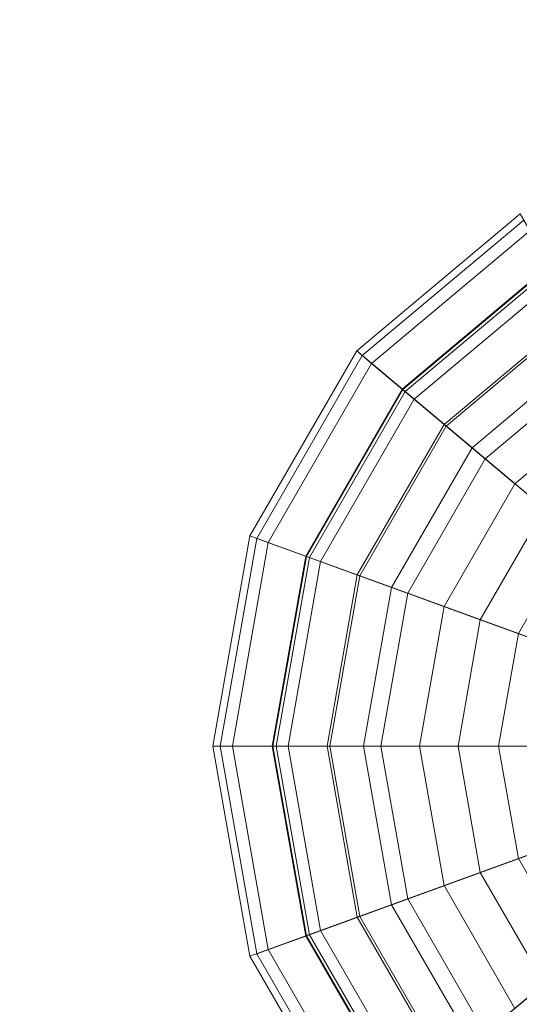
# Model space of a CAD drawing. Units: inches. Extents: x 375 to 1122, y 27 to 1069.
# Tile 109 of 155: x 731.282 to 732.383, y 872.701 to 874.871. Entities that reach past the tile are written whole.
import ezdxf

# ---------------------------------------------------------------- set-up
doc = ezdxf.new("R2010")
doc.units = ezdxf.units.IN
doc.layers.add('A-ANNO-DIMS', color=2, linetype='Continuous', lineweight=18)
doc.layers.add('Furniture', color=30, linetype='Continuous', lineweight=18)
doc.styles.get("Standard").update_dxf_attribs({"font": 'arial.ttf'})
doc.dimstyles.new('ISO-25', dxfattribs={"dimtxt": 12, "dimasz": 2.5, "dimexe": 1.5, "dimexo": 1.5, "dimtad": 1, "dimdec": 1, "dimlunit": 3, "dimtxsty": 'Standard', "dimblk": 'ARCHTICK', "dimcen": 2.5, "dimadec": 0, "dimazin": 0, "dimtfac": 1, "dimtdec": 1, "dimtmove": 0, "dimatfit": 3, "dimfxl": 1.5, "dimfxlon": 1, "dimarcsym": 0})

# ---------------------------------------------------------------- blocks, each defined once
blk = doc.blocks.new('A$C403C54AD')
for points in [[(1.597139, 1.185986, -0.04658), (1.626464, 1.202917, -0.043501), (1.626464, 1.202917, -0.043501), (1.604698, 1.176977, -0.04658)], [(1.604698, 1.176977, -0.04658), (1.626464, 1.202917, -0.043501), (1.626464, 1.202917, -0.043501), (1.614883, 1.171097, -0.04658)], [(1.614883, 1.171097, -0.04658), (1.626464, 1.202917, -0.043501), (1.626464, 1.202917, -0.043501), (1.626464, 1.169055, -0.04658)], [(1.64823, 1.176977, -0.04658), (1.626464, 1.202917, -0.043501), (1.626464, 1.202917, -0.043501), (1.65579, 1.185986, -0.04658)], [(1.638046, 1.171097, -0.04658), (1.626464, 1.202917, -0.043501), (1.626464, 1.202917, -0.043501), (1.64823, 1.176977, -0.04658)], [(1.626464, 1.169055, -0.04658), (1.626464, 1.202917, -0.043501), (1.626464, 1.202917, -0.043501), (1.638046, 1.171097, -0.04658)], [(1.620741, 1.196096, 0.042248), (1.614812, 1.189031, 0.048884), (1.620264, 1.185883, 0.048884), (1.623419, 1.19455, 0.042248)], [(1.62951, 1.19455, 0.042248), (1.632664, 1.185883, 0.048884), (1.638116, 1.189031, 0.048884), (1.632188, 1.196096, 0.042248)], [(1.614154, 1.19581, -0.040074), (1.599967, 1.187619, -0.043349), (1.606797, 1.179479, -0.043349), (1.617327, 1.192029, -0.040074)], [(1.635601, 1.192029, -0.040074), (1.646131, 1.179479, -0.043349), (1.652961, 1.187619, -0.043349), (1.638774, 1.19581, -0.040074)], [(1.613379, 1.187323, 0.046697), (1.61996, 1.195166, 0.03933), (1.623003, 1.193409, 0.03933), (1.619501, 1.183788, 0.046697)], [(1.633427, 1.183788, 0.046697), (1.629925, 1.193409, 0.03933), (1.632968, 1.195166, 0.03933), (1.63955, 1.187323, 0.046697)], [(1.623419, 1.19455, 0.042248), (1.620264, 1.185883, 0.048884), (1.626464, 1.18479, 0.048884), (1.626464, 1.194013, 0.042248)], [(1.626464, 1.194013, 0.042248), (1.626464, 1.18479, 0.048884), (1.632664, 1.185883, 0.048884), (1.62951, 1.19455, 0.042248)], [(1.610766, 1.193854, 0.048884), (1.605149, 1.190611, 0.058276), (1.610643, 1.184063, 0.058276), (1.614812, 1.189031, 0.048884)], [(1.619501, 1.183788, 0.046697), (1.623003, 1.193409, 0.03933), (1.626464, 1.192799, 0.03933), (1.626464, 1.18256, 0.046697)], [(1.626464, 1.18256, 0.046697), (1.626464, 1.192799, 0.03933), (1.629925, 1.193409, 0.03933), (1.633427, 1.183788, 0.046697)], [(1.638116, 1.189031, 0.048884), (1.642285, 1.184063, 0.058276), (1.64778, 1.190611, 0.058276), (1.642163, 1.193854, 0.048884)], [(1.602714, 1.189206, 0.056929), (1.608834, 1.192739, 0.046697), (1.613379, 1.187323, 0.046697), (1.608836, 1.18191, 0.056929)], [(1.644092, 1.18191, 0.056929), (1.63955, 1.187323, 0.046697), (1.644094, 1.192739, 0.046697), (1.650214, 1.189206, 0.056929)], [(1.617327, 1.192029, -0.040074), (1.606797, 1.179479, -0.043349), (1.616, 1.174166, -0.043349), (1.621603, 1.18956, -0.040074)], [(1.631326, 1.18956, -0.040074), (1.636929, 1.174166, -0.043349), (1.646131, 1.179479, -0.043349), (1.635601, 1.192029, -0.040074)], [(1.602589, 1.189133, 0.115599), (1.606995, 1.191677, 0.12581), (1.612014, 1.185696, 0.12581), (1.608743, 1.181798, 0.115599)], [(1.606995, 1.191677, 0.12581), (1.604329, 1.190138, 0.12581), (1.610035, 1.183338, 0.12581), (1.612014, 1.185696, 0.12581)], [(1.604329, 1.190138, 0.12581), (1.600002, 1.187639, 0.116404), (1.606823, 1.17951, 0.116404), (1.610035, 1.183338, 0.12581)], [(1.605149, 1.190611, 0.058276), (1.600725, 1.188057, 0.075423), (1.60736, 1.18015, 0.075423), (1.610643, 1.184063, 0.058276)], [(1.621603, 1.18956, -0.040074), (1.616, 1.174166, -0.043349), (1.626464, 1.172321, -0.043349), (1.626464, 1.188703, -0.040074)], [(1.626464, 1.188703, -0.040074), (1.626464, 1.172321, -0.043349), (1.636929, 1.174166, -0.043349), (1.631326, 1.18956, -0.040074)], [(1.598069, 1.186523, 0.074938), (1.602714, 1.189206, 0.056929), (1.608836, 1.18191, 0.056929), (1.605388, 1.1778, 0.074938)], [(1.600155, 1.187728, 0.102963), (1.602589, 1.189133, 0.115599), (1.608743, 1.181798, 0.115599), (1.606937, 1.179646, 0.102963)], [(1.614812, 1.189031, 0.048884), (1.610643, 1.184063, 0.058276), (1.618046, 1.179789, 0.058276), (1.620264, 1.185883, 0.048884)], [(1.632664, 1.185883, 0.048884), (1.634882, 1.179789, 0.058276), (1.642285, 1.184063, 0.058276), (1.638116, 1.189031, 0.048884)], [(1.600725, 1.188057, 0.075423), (1.600155, 1.187728, 0.102963), (1.606937, 1.179646, 0.102963), (1.60736, 1.18015, 0.075423)], [(1.599967, 1.187619, -0.043349), (1.597139, 1.185986, -0.04658), (1.604698, 1.176977, -0.04658), (1.606797, 1.179479, -0.043349)], [(1.600002, 1.187639, 0.116404), (1.597484, 1.186186, 0.10318), (1.604954, 1.177283, 0.10318), (1.606823, 1.17951, 0.116404)], [(1.608836, 1.18191, 0.056929), (1.613379, 1.187323, 0.046697), (1.619501, 1.183788, 0.046697), (1.617085, 1.177147, 0.056929)], [(1.635844, 1.177147, 0.056929), (1.633427, 1.183788, 0.046697), (1.63955, 1.187323, 0.046697), (1.644092, 1.18191, 0.056929)], [(1.597484, 1.186186, 0.10318), (1.598069, 1.186523, 0.074938), (1.605388, 1.1778, 0.074938), (1.604954, 1.177283, 0.10318)], [(1.620264, 1.185883, 0.048884), (1.618046, 1.179789, 0.058276), (1.626464, 1.178304, 0.058276), (1.626464, 1.18479, 0.048884)], [(1.626464, 1.18479, 0.048884), (1.626464, 1.178304, 0.058276), (1.634882, 1.179789, 0.058276), (1.632664, 1.185883, 0.048884)], [(1.608743, 1.181798, 0.115599), (1.612014, 1.185696, 0.12581), (1.618775, 1.181792, 0.12581), (1.617035, 1.177011, 0.115599)], [(1.612014, 1.185696, 0.12581), (1.610035, 1.183338, 0.12581), (1.617722, 1.178899, 0.12581), (1.618775, 1.181792, 0.12581)], [(1.634153, 1.181792, 0.12581), (1.635206, 1.178899, 0.12581), (1.642894, 1.183338, 0.12581), (1.640915, 1.185696, 0.12581)], [(1.635893, 1.177011, 0.115599), (1.634153, 1.181792, 0.12581), (1.640915, 1.185696, 0.12581), (1.644185, 1.181798, 0.115599)], [(1.610643, 1.184063, 0.058276), (1.60736, 1.18015, 0.075423), (1.616299, 1.174989, 0.075423), (1.618046, 1.179789, 0.058276)], [(1.617085, 1.177147, 0.056929), (1.619501, 1.183788, 0.046697), (1.626464, 1.18256, 0.046697), (1.626464, 1.175494, 0.056929)], [(1.626464, 1.175494, 0.056929), (1.626464, 1.18256, 0.046697), (1.633427, 1.183788, 0.046697), (1.635844, 1.177147, 0.056929)], [(1.634882, 1.179789, 0.058276), (1.636629, 1.174989, 0.075423), (1.645568, 1.18015, 0.075423), (1.642285, 1.184063, 0.058276)], [(1.610035, 1.183338, 0.12581), (1.606823, 1.17951, 0.116404), (1.616013, 1.174204, 0.116404), (1.617722, 1.178899, 0.12581)], [(1.635206, 1.178899, 0.12581), (1.636915, 1.174204, 0.116404), (1.646105, 1.17951, 0.116404), (1.642894, 1.183338, 0.12581)], [(1.605388, 1.1778, 0.074938), (1.608836, 1.18191, 0.056929), (1.617085, 1.177147, 0.056929), (1.61525, 1.172106, 0.074938)], [(1.606937, 1.179646, 0.102963), (1.608743, 1.181798, 0.115599), (1.617035, 1.177011, 0.115599), (1.616074, 1.174371, 0.102963)], [(1.617035, 1.177011, 0.115599), (1.618775, 1.181792, 0.12581), (1.626464, 1.180436, 0.12581), (1.626464, 1.175348, 0.115599)], [(1.618775, 1.181792, 0.12581), (1.617722, 1.178899, 0.12581), (1.626464, 1.177358, 0.12581), (1.626464, 1.180436, 0.12581)], [(1.626464, 1.180436, 0.12581), (1.626464, 1.177358, 0.12581), (1.635206, 1.178899, 0.12581), (1.634153, 1.181792, 0.12581)], [(1.626464, 1.175348, 0.115599), (1.626464, 1.180436, 0.12581), (1.634153, 1.181792, 0.12581), (1.635893, 1.177011, 0.115599)], [(1.637678, 1.172106, 0.074938), (1.635844, 1.177147, 0.056929), (1.644092, 1.18191, 0.056929), (1.64754, 1.1778, 0.074938)], [(1.636854, 1.174371, 0.102963), (1.635893, 1.177011, 0.115599), (1.644185, 1.181798, 0.115599), (1.645991, 1.179646, 0.102963)], [(1.60736, 1.18015, 0.075423), (1.606937, 1.179646, 0.102963), (1.616074, 1.174371, 0.102963), (1.616299, 1.174989, 0.075423)], [(1.636629, 1.174989, 0.075423), (1.636854, 1.174371, 0.102963), (1.645991, 1.179646, 0.102963), (1.645568, 1.18015, 0.075423)], [(1.606797, 1.179479, -0.043349), (1.604698, 1.176977, -0.04658), (1.614883, 1.171097, -0.04658), (1.616, 1.174166, -0.043349)], [(1.606823, 1.17951, 0.116404), (1.604954, 1.177283, 0.10318), (1.615019, 1.171472, 0.10318), (1.616013, 1.174204, 0.116404)], [(1.618046, 1.179789, 0.058276), (1.616299, 1.174989, 0.075423), (1.626464, 1.173197, 0.075423), (1.626464, 1.178304, 0.058276)], [(1.626464, 1.178304, 0.058276), (1.626464, 1.173197, 0.075423), (1.636629, 1.174989, 0.075423), (1.634882, 1.179789, 0.058276)], [(1.636915, 1.174204, 0.116404), (1.637909, 1.171472, 0.10318), (1.647974, 1.177283, 0.10318), (1.646105, 1.17951, 0.116404)], [(1.636929, 1.174166, -0.043349), (1.638046, 1.171097, -0.04658), (1.64823, 1.176977, -0.04658), (1.646131, 1.179479, -0.043349)], [(1.617722, 1.178899, 0.12581), (1.616013, 1.174204, 0.116404), (1.626464, 1.172361, 0.116404), (1.626464, 1.177358, 0.12581)], [(1.626464, 1.177358, 0.12581), (1.626464, 1.172361, 0.116404), (1.636915, 1.174204, 0.116404), (1.635206, 1.178899, 0.12581)], [(1.604954, 1.177283, 0.10318), (1.605388, 1.1778, 0.074938), (1.61525, 1.172106, 0.074938), (1.615019, 1.171472, 0.10318)], [(1.637909, 1.171472, 0.10318), (1.637678, 1.172106, 0.074938), (1.64754, 1.1778, 0.074938), (1.647974, 1.177283, 0.10318)], [(1.61525, 1.172106, 0.074938), (1.617085, 1.177147, 0.056929), (1.626464, 1.175494, 0.056929), (1.626464, 1.170129, 0.074938)], [(1.626464, 1.170129, 0.074938), (1.626464, 1.175494, 0.056929), (1.635844, 1.177147, 0.056929), (1.637678, 1.172106, 0.074938)], [(1.616074, 1.174371, 0.102963), (1.617035, 1.177011, 0.115599), (1.626464, 1.175348, 0.115599), (1.626464, 1.172539, 0.102963)], [(1.626464, 1.172539, 0.102963), (1.626464, 1.175348, 0.115599), (1.635893, 1.177011, 0.115599), (1.636854, 1.174371, 0.102963)], [(1.616299, 1.174989, 0.075423), (1.616074, 1.174371, 0.102963), (1.626464, 1.172539, 0.102963), (1.626464, 1.173197, 0.075423)], [(1.626464, 1.173197, 0.075423), (1.626464, 1.172539, 0.102963), (1.636854, 1.174371, 0.102963), (1.636629, 1.174989, 0.075423)], [(1.616, 1.174166, -0.043349), (1.614883, 1.171097, -0.04658), (1.626464, 1.169055, -0.04658), (1.626464, 1.172321, -0.043349)], [(1.616013, 1.174204, 0.116404), (1.615019, 1.171472, 0.10318), (1.626464, 1.169454, 0.10318), (1.626464, 1.172361, 0.116404)], [(1.626464, 1.172361, 0.116404), (1.626464, 1.169454, 0.10318), (1.637909, 1.171472, 0.10318), (1.636915, 1.174204, 0.116404)], [(1.626464, 1.172321, -0.043349), (1.626464, 1.169055, -0.04658), (1.638046, 1.171097, -0.04658), (1.636929, 1.174166, -0.043349)], [(1.615019, 1.171472, 0.10318), (1.61525, 1.172106, 0.074938), (1.626464, 1.170129, 0.074938), (1.626464, 1.169454, 0.10318)], [(1.626464, 1.169454, 0.10318), (1.626464, 1.170129, 0.074938), (1.637678, 1.172106, 0.074938), (1.637909, 1.171472, 0.10318)]]:
    blk.add_3dface(points)
blk = doc.blocks.new('_ArchTick')
at = {"color": 0, "linetype": 'ByBlock', "const_width": 0.15}
blk.add_lwpolyline([(-0.5, -0.5), (0.5, 0.5)], dxfattribs=at)
blk = doc.blocks.new('*D88')
at = {"layer": 'A-ANNO-DIMS', "color": 0, "lineweight": -2, "transparency": 16777216}
for p, q in [((731.0073, 1052.5277), (731.0073, 1055.5277)), ((854.0073, 1052.5277), (854.0073, 1055.5277)), ((731.0073, 1054.0277), (854.0073, 1054.0277))]:
    blk.add_line(p, q, dxfattribs=at)
at = {"layer": 'Defpoints', "color": 0, "transparency": 16777216}
for p in [(854.0073, 1054.0277), (731.0073, 502.5277), (854.0073, 502.5277)]:
    blk.add_point(p, dxfattribs=at)
at = {"layer": 'A-ANNO-DIMS', "color": 0, "lineweight": -2, "transparency": 16777216, "xscale": 2.5, "yscale": 2.5, "zscale": 2.5, "rotation": 180}
blk.add_blockref('_ArchTick', (731.0073, 1054.0277), dxfattribs=at)
at = {"layer": 'A-ANNO-DIMS', "color": 0, "lineweight": -2, "transparency": 16777216, "xscale": 2.5, "yscale": 2.5, "zscale": 2.5}
blk.add_blockref('_ArchTick', (854.0073, 1054.0277), dxfattribs=at)
at = {"layer": 'A-ANNO-DIMS', "color": 0, "transparency": 16777216, "insert": (792.5073, 1060.7837), "char_height": 12, "attachment_point": 5}
blk.add_mtext('10\'-3"', dxfattribs=at)
blk = doc.blocks.new('*D91')
at = {"layer": 'A-ANNO-DIMS', "color": 0, "lineweight": -2, "transparency": 16777216}
for p, q in [((728.0073, 1052.5277), (728.0073, 1055.5277)), ((788.0073, 1052.5277), (788.0073, 1055.5277)), ((728.0073, 1054.0277), (788.0073, 1054.0277))]:
    blk.add_line(p, q, dxfattribs=at)
at = {"layer": 'Defpoints', "color": 0, "transparency": 16777216}
for p in [(788.0073, 1054.0277), (728.0073, 774.0277), (788.0073, 774.0277)]:
    blk.add_point(p, dxfattribs=at)
at = {"layer": 'A-ANNO-DIMS', "color": 0, "lineweight": -2, "transparency": 16777216, "xscale": 2.5, "yscale": 2.5, "zscale": 2.5, "rotation": 180}
blk.add_blockref('_ArchTick', (728.0073, 1054.0277), dxfattribs=at)
at = {"layer": 'A-ANNO-DIMS', "color": 0, "lineweight": -2, "transparency": 16777216, "xscale": 2.5, "yscale": 2.5, "zscale": 2.5}
blk.add_blockref('_ArchTick', (788.0073, 1054.0277), dxfattribs=at)
at = {"layer": 'A-ANNO-DIMS', "color": 0, "transparency": 16777216, "insert": (758.0073, 1060.7796), "char_height": 12, "attachment_point": 5}
blk.add_mtext('5\'-0"', dxfattribs=at)

msp = doc.modelspace()

# ---------------------------------------------------------------- block references
at = {"layer": 'Furniture', "xscale": 39.9918517141215, "yscale": 39.9918517141215, "zscale": 39.9918517141215, "rotation": 270}
msp.add_blockref('A$C403C54AD', (684.9549, 938.3156, 0.024), dxfattribs=at)

# ---------------------------------------------------------------- dimensions: what is measured, and where the dimension line sits
at = {"layer": 'A-ANNO-DIMS'}
for base, p1, p2, picture, middle in [((788.0073, 1054.0277), (728.0073, 774.0277), (788.0073, 774.0277), '*D91', (758.0073, 1060.7796)), ((854.0073, 1054.0277), (731.0073, 502.5277), (854.0073, 502.5277), '*D88', (792.5073, 1060.7837))]:
    dim = msp.add_linear_dim(base=base, p1=p1, p2=p2, dimstyle='ISO-25', override={"dimdec": 1, "dimlfac": 1, "dimrnd": 0, "dimzin": 1, "dimdsep": 46, "dimlunit": 4, "dimfrac": 2}, dxfattribs=at)
    dim.commit()
    dim.dimension.update_dxf_attribs({"geometry": picture, "text_midpoint": middle})

doc.saveas('drawing.dxf')
